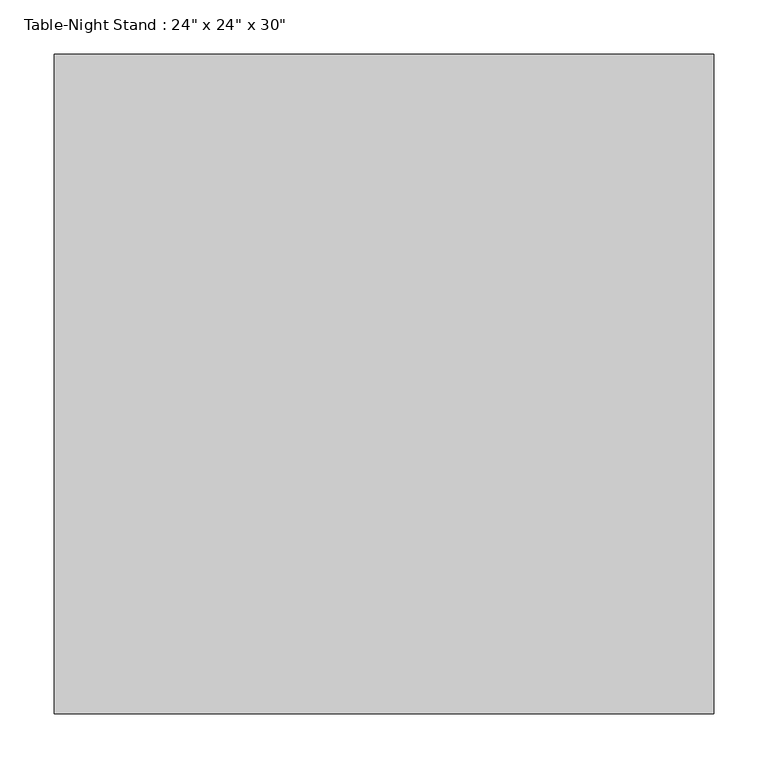
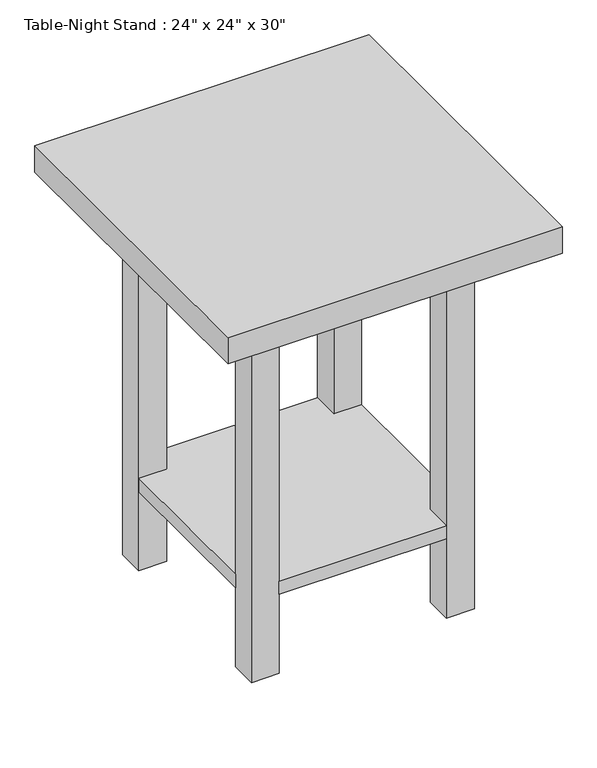
"""IFC4 building model written with IfcOpenShell, lengths in millimetres: furniture geometry."""

from ifc_helpers import new_model, si_unit, frame, origin, origin_with_axes, place, context, project, spatial, polyline, outline, extrude, source, transform, mapped, element, save


def furniture_5bc9ed15(model_context):
    return source(origin(), model_context, "Body", "SweptSolid", [
        extrude(outline(polyline([(156.1336303, 508.0), (460.9336303, 508.0), (460.9336303, 457.2), (511.7336303, 457.2), (511.7336303, 152.4), (460.9336303, 152.4), (460.9336303, 101.6), (156.1336303, 101.6), (156.1336303, 152.4), (105.3336303, 152.4), (105.3336303, 457.2), (156.1336303, 457.2), (156.1336303, 508.0)])), frame((0.0, 0.0, 152.4), z_axis=(0.0, 0.0, 1.0), x_axis=(1.0, 0.0, 0.0)), (0.0, 0.0, 1.0), 25.4),
        extrude(outline(polyline([(156.1336303, 508.0), (156.1336303, 457.2), (105.3336303, 457.2), (105.3336303, 508.0), (156.1336303, 508.0)])), origin_with_axes(), (0.0, 0.0, 1.0), 711.2),
        extrude(outline(polyline([(156.1336303, 152.4), (156.1336303, 101.6), (105.3336303, 101.6), (105.3336303, 152.4), (156.1336303, 152.4)])), origin_with_axes(), (0.0, 0.0, 1.0), 711.2),
        extrude(outline(polyline([(511.7336303, 508.0), (511.7336303, 457.2), (460.9336303, 457.2), (460.9336303, 508.0), (511.7336303, 508.0)])), origin_with_axes(), (0.0, 0.0, 1.0), 711.2),
        extrude(outline(polyline([(511.7336303, 152.4), (511.7336303, 101.6), (460.9336303, 101.6), (460.9336303, 152.4), (511.7336303, 152.4)])), origin_with_axes(), (0.0, 0.0, 1.0), 711.2),
        extrude(outline(polyline([(613.3336303, 0.0), (3.7336303, 0.0), (3.7336303, 609.6), (613.3336303, 609.6), (613.3336303, 0.0)])), frame((0.0, 0.0, 711.2), z_axis=(0.0, 0.0, 1.0), x_axis=(1.0, 0.0, 0.0)), (0.0, 0.0, 1.0), 50.8),
    ])


if __name__ == "__main__":
    model = new_model("IFC4")
    model_context = context("Model", 3, world=origin())
    ifc_project = project(units=[si_unit("LENGTHUNIT", "METRE", prefix="MILLI")], contexts=[model_context])
    site = spatial("IfcSite", under=ifc_project)
    building = spatial("IfcBuilding", under=site)
    placement = place(None, origin())
    furniture_shape = furniture_5bc9ed15(model_context)
    element("IfcFurniture", 1, ObjectType="Table-Night Stand : 24\" x 24\" x 30\"", at=placement, inside=building, context=model_context, shape_type="MappedRepresentation", body=[
        mapped(furniture_shape, transform((0.0, 0.0, 0.0), x_axis=(1.0, 0.0, 0.0), y_axis=(0.0, 1.0, 0.0), z_axis=(0.0, 0.0, 1.0))),
    ])
    save(model, "model.ifc")

# Revit data of these elements
# Type "Table-Night Stand : 24\" x 24\" x 30\""
#   Assembly Code = "E2020200"
#   Depth = 2' - 0"
#   Height = 2' - 6"
#   Width = 2' - 0"
#   Base Material = Birch
#   Top Material = Laminate, Ivory, Matte
#   Default Elevation = 0
# Element 1 (IfcFurniture, "Table-Night Stand : 24\" x 24\" x 30\"")
#   Materials on its faces: "Birch", "Laminate, Ivory, Matte"
# Materials
#   "Birch": class "Wood", colour RGB 224 178 126, transparency 0, Description = "Betula Alleghaniensis", Cost = 0
#   "Laminate, Ivory, Matte": class "Plastic", colour RGB 247 247 239, transparency 0, Description = "Plastic Laminate - Ivory, Matte", Cost = 0
